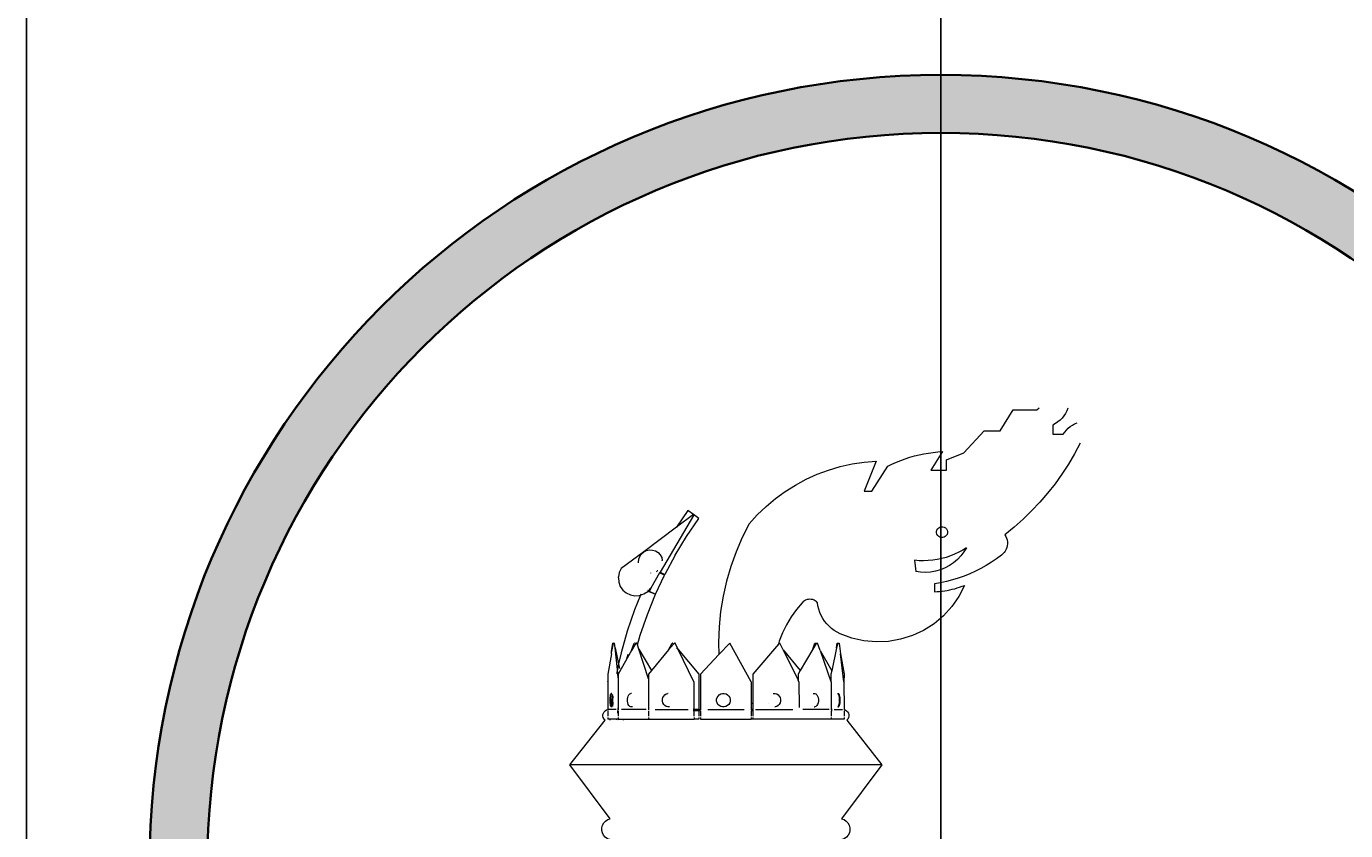
# Model space of a CAD drawing. Units: millimetres. Extents: x 446512 to 447461, y 70395 to 70610.
# Tile 30 of 39: x 447255 to 447300, y 70477 to 70505. Entities that reach past the tile are written whole.
import ezdxf

# ---------------------------------------------------------------- set-up
doc = ezdxf.new("R2010")
doc.units = ezdxf.units.MM
for name, color, linetype, lineweight in [('A-ANNO-DIMS', 2, 'Continuous', 18), ('A-FURN', 7, 'Continuous', 35), ('A-FURN-DECO', 8, 'Continuous', 13), ('A-FURN-PATT', 38, 'Continuous', 13)]:
    doc.layers.add(name, color=color, linetype=linetype, lineweight=lineweight)
doc.styles.get("Standard").update_dxf_attribs({"font": 'arial.ttf'})
doc.dimstyles.get("Standard").update_dxf_attribs({"dimtxt": 0.18, "dimasz": 0.18, "dimexe": 0.18, "dimexo": 0.0625, "dimgap": 0.09, "dimtad": 0, "dimtih": 1, "dimtoh": 1, "dimdec": 4, "dimzin": 0, "dimdsep": 46, "dimtxsty": 'Standard', "dimcen": 0.09, "dimadec": 0, "dimazin": 0, "dimtfac": 1, "dimtdec": 4, "dimtofl": 0, "dimtmove": 0, "dimatfit": 3, "dimfxl": 1, "dimtolj": 1, "dimtzin": 0, "dimarcsym": 0})

# ---------------------------------------------------------------- blocks, each defined once
blk = doc.blocks.new('DECO-SCULPTURE-BIRD')
for p, q in [((15.181, 34.03), (15.627, 34.749)), ((15.627, 34.749), (16.449, 34.749)), ((16.449, 34.749), (16.526, 34.819)), ((13.93, 33.268), (14.629, 34.03)), ((14.629, 34.03), (15.181, 34.03)), ((12.541, 33.233), (12.703, 33.261)), ((12.703, 33.261), (12.866, 33.283)), ((13.195, 33.309), (12.789, 32.676)), ((12.866, 33.283), (13.03, 33.299)), ((13.03, 33.299), (13.195, 33.309)), ((13.33, 33.029), (13.93, 33.268)), ((17.942, 33.598), (17.748, 33.234)), ((9.257, 32.674), (9.658, 32.793)), ((9.658, 32.793), (10.067, 32.884)), ((10.067, 32.884), (10.481, 32.948)), ((10.481, 32.948), (10.898, 32.983)), ((10.898, 32.983), (10.488, 31.945)), ((10.747, 31.945), (11.298, 32.806)), ((11.298, 32.806), (11.446, 32.878)), ((11.446, 32.878), (11.597, 32.946)), ((11.597, 32.946), (11.749, 33.008)), ((11.749, 33.008), (11.904, 33.064)), ((11.904, 33.064), (12.061, 33.115)), ((12.061, 33.115), (12.219, 33.16)), ((12.219, 33.16), (12.379, 33.199)), ((12.379, 33.199), (12.541, 33.233)), ((13.33, 32.676), (13.33, 33.029)), ((17.539, 32.879), (17.314, 32.533)), ((17.748, 33.234), (17.539, 32.879)), ((8.113, 32.157), (8.482, 32.355)), ((8.482, 32.355), (8.864, 32.528)), ((8.864, 32.528), (9.257, 32.674)), ((12.789, 32.676), (13.33, 32.676)), ((17.314, 32.533), (17.074, 32.198)), ((7.42, 31.689), (7.759, 31.935)), ((7.759, 31.935), (8.113, 32.157)), ((10.488, 31.945), (10.747, 31.945)), ((17.074, 32.198), (16.819, 31.874)), ((6.796, 31.131), (7.098, 31.42)), ((7.098, 31.42), (7.42, 31.689)), ((16.55, 31.562), (16.267, 31.262)), ((16.819, 31.874), (16.55, 31.562)), ((4.59, 31.11), (3.442, 29.152)), ((4.396, 31.274), (4.005, 30.703)), ((4.59, 31.141), (4.005, 30.703)), ((4.354, 30.38), (4.784, 31.008)), ((4.59, 31.141), (4.396, 31.274)), ((4.59, 31.11), (4.59, 31.141)), ((4.784, 31.008), (4.59, 31.141)), ((6.514, 30.821), (6.796, 31.131)), ((15.971, 30.975), (15.663, 30.701)), ((16.267, 31.262), (15.971, 30.975)), ((4.005, 30.703), (2.875, 29.852)), ((6.514, 30.821), (6.273, 30.344)), ((15.663, 30.701), (15.342, 30.442)), ((3.962, 29.736), (4.354, 30.38)), ((6.273, 30.344), (6.062, 29.854)), ((15.342, 30.442), (15.375, 30.385)), ((15.375, 30.385), (15.4, 30.324)), ((15.4, 30.324), (15.418, 30.261)), ((15.422, 30.065), (15.408, 30.001)), ((15.418, 30.261), (15.428, 30.196)), ((15.429, 30.13), (15.422, 30.065)), ((15.428, 30.196), (15.429, 30.13)), ((2.875, 29.852), (2.1, 29.278)), ((2.704, 29.597), (2.737, 29.696)), ((2.737, 29.696), (2.795, 29.783)), ((2.795, 29.783), (2.875, 29.852)), ((2.875, 29.852), (2.971, 29.899)), ((2.971, 29.899), (3.076, 29.921)), ((3.076, 29.921), (3.183, 29.915)), ((3.183, 29.915), (3.285, 29.883)), ((3.285, 29.883), (3.375, 29.827)), ((3.375, 29.827), (3.447, 29.75)), ((3.447, 29.75), (3.496, 29.657)), ((3.496, 29.657), (3.518, 29.556)), ((3.962, 29.736), (3.605, 29.071)), ((6.062, 29.854), (5.881, 29.351)), ((15.054, 29.609), (14.878, 29.491)), ((15.224, 29.735), (15.054, 29.609)), ((15.274, 29.778), (15.224, 29.735)), ((15.318, 29.827), (15.274, 29.778)), ((15.355, 29.881), (15.318, 29.827)), ((15.385, 29.939), (15.355, 29.881)), ((15.408, 30.001), (15.385, 29.939)), ((2.1, 29.278), (2.031, 29.139)), ((2.698, 29.494), (2.704, 29.597)), ((2.699, 29.49), (2.698, 29.494)), ((2.698, 29.476), (2.699, 29.49)), ((3.306, 29.18), (3.325, 29.171)), ((3.358, 29.194), (3.345, 29.201)), ((3.442, 29.152), (3.425, 29.125)), ((3.442, 29.152), (3.605, 29.071)), ((3.517, 29.541), (3.518, 29.556)), ((3.517, 29.541), (3.518, 29.538)), ((5.881, 29.351), (5.732, 28.838)), ((14.324, 29.181), (14.131, 29.094)), ((14.513, 29.277), (14.324, 29.181)), ((14.698, 29.38), (14.513, 29.277)), ((14.878, 29.491), (14.698, 29.38)), ((2.031, 29.139), (2.002, 28.989)), ((2.002, 28.958), (2.002, 28.989)), ((2.002, 28.958), (2.013, 28.805)), ((2.013, 28.805), (2.066, 28.66)), ((3.425, 29.125), (3.119, 28.602)), ((3.287, 28.392), (3.593, 29.046)), ((3.593, 29.046), (3.425, 29.125)), ((5.732, 28.838), (5.615, 28.317)), ((13.121, 28.783), (12.912, 28.746)), ((12.912, 28.746), (12.912, 28.476)), ((13.328, 28.828), (13.121, 28.783)), ((13.532, 28.882), (13.328, 28.828)), ((13.735, 28.944), (13.532, 28.882)), ((13.934, 29.015), (13.735, 28.944)), ((13.947, 28.695), (13.752, 28.315)), ((13.864, 28.663), (13.947, 28.695)), ((14.131, 29.094), (13.934, 29.015)), ((2.066, 28.66), (2.155, 28.533)), ((2.155, 28.533), (2.275, 28.433)), ((2.275, 28.433), (2.419, 28.366)), ((2.419, 28.366), (2.575, 28.337)), ((2.766, 28.36), (2.561, 27.852)), ((2.575, 28.337), (2.733, 28.349)), ((2.733, 28.349), (2.766, 28.36)), ((2.766, 28.36), (2.883, 28.399)), ((2.781, 28.395), (2.766, 28.36)), ((2.883, 28.399), (3.015, 28.486)), ((3.002, 27.688), (3.284, 28.387)), ((3.005, 28.509), (3.027, 28.499)), ((3.015, 28.486), (3.027, 28.499)), ((3.036, 28.509), (3.019, 28.518)), ((3.027, 28.499), (3.036, 28.509)), ((3.027, 28.499), (3.284, 28.387)), ((3.036, 28.509), (3.119, 28.602)), ((3.036, 28.509), (3.287, 28.392)), ((3.074, 28.492), (3.069, 28.481)), ((3.152, 28.659), (3.074, 28.492)), ((5.615, 28.317), (5.531, 27.79)), ((12.912, 28.476), (13.001, 28.48)), ((13.001, 28.48), (13.089, 28.487)), ((13.089, 28.487), (13.177, 28.496)), ((13.177, 28.496), (13.265, 28.508)), ((13.265, 28.508), (13.352, 28.523)), ((13.352, 28.523), (13.439, 28.54)), ((13.439, 28.54), (13.525, 28.559)), ((13.752, 28.315), (13.509, 27.964)), ((13.525, 28.559), (13.611, 28.581)), ((13.611, 28.581), (13.696, 28.606)), ((13.696, 28.606), (13.781, 28.633)), ((13.781, 28.633), (13.864, 28.663)), ((2.561, 27.852), (2.308, 27.114)), ((5.531, 27.79), (5.479, 27.259)), ((8.147, 27.859), (7.968, 27.605)), ((8.346, 28.098), (8.147, 27.859)), ((8.382, 28.133), (8.346, 28.098)), ((8.422, 28.162), (8.382, 28.133)), ((8.466, 28.185), (8.422, 28.162)), ((8.513, 28.202), (8.466, 28.185)), ((8.561, 28.212), (8.513, 28.202)), ((8.611, 28.216), (8.561, 28.212)), ((8.66, 28.212), (8.611, 28.216)), ((8.709, 28.202), (8.66, 28.212)), ((8.756, 28.185), (8.709, 28.202)), ((8.799, 28.162), (8.756, 28.185)), ((8.84, 28.133), (8.799, 28.162)), ((8.875, 28.098), (8.84, 28.133)), ((8.892, 27.984), (8.875, 28.098)), ((8.919, 27.871), (8.892, 27.984)), ((8.956, 27.761), (8.919, 27.871)), ((13.509, 27.964), (13.223, 27.648)), ((2.757, 26.974), (3.002, 27.688)), ((7.808, 27.338), (7.671, 27.059)), ((7.968, 27.605), (7.808, 27.338)), ((9.002, 27.655), (8.956, 27.761)), ((9.057, 27.553), (9.002, 27.655)), ((9.121, 27.456), (9.057, 27.553)), ((9.193, 27.366), (9.121, 27.456)), ((9.273, 27.282), (9.193, 27.366)), ((12.897, 27.372), (12.537, 27.142)), ((13.223, 27.648), (12.897, 27.372)), ((2.308, 27.114), (2.095, 26.364)), ((2.662, 26.638), (2.757, 26.974)), ((5.479, 27.259), (5.46, 26.725)), ((7.671, 27.059), (7.556, 26.77)), ((9.359, 27.205), (9.273, 27.282)), ((9.452, 27.136), (9.359, 27.205)), ((9.551, 27.075), (9.452, 27.136)), ((9.654, 27.023), (9.551, 27.075)), ((10.055, 26.875), (9.654, 27.023)), ((10.471, 26.78), (10.055, 26.875)), ((12.15, 26.961), (11.743, 26.833)), ((12.537, 27.142), (12.15, 26.961)), ((1.77, 26.41), (1.808, 26.703)), ((1.827, 26.703), (1.77, 26.41)), ((1.827, 26.703), (1.808, 26.703)), ((1.827, 26.703), (1.873, 26.703)), ((1.89, 26.535), (1.873, 26.703)), ((1.89, 26.535), (2.01, 25.987)), ((1.967, 25.795), (1.89, 26.535)), ((2.459, 26.45), (1.998, 25.636)), ((2.459, 26.45), (2.547, 26.703)), ((2.603, 26.703), (2.459, 26.45)), ((2.558, 26.703), (2.547, 26.703)), ((2.64, 26.703), (2.603, 26.703)), ((2.662, 26.638), (2.64, 26.703)), ((2.709, 26.493), (2.662, 26.638)), ((2.709, 26.493), (3.149, 25.76)), ((3.046, 25.467), (2.709, 26.493)), ((3.737, 26.466), (3.149, 25.76)), ((3.737, 26.466), (3.854, 26.703)), ((3.905, 26.667), (3.737, 26.466)), ((3.875, 26.703), (3.854, 26.703)), ((3.875, 26.703), (3.905, 26.667)), ((3.935, 26.703), (3.905, 26.667)), ((3.957, 26.703), (3.935, 26.703)), ((4.064, 26.48), (3.957, 26.703)), ((4.013, 26.541), (4.064, 26.48)), ((4.064, 26.48), (4.783, 25.636)), ((4.603, 25.364), (4.064, 26.48)), ((5.46, 26.725), (5.471, 26.308)), ((5.845, 26.703), (5.471, 26.308)), ((6.58, 25.364), (5.845, 26.703)), ((7.523, 26.665), (6.643, 25.636)), ((7.523, 26.665), (7.514, 26.636)), ((7.526, 26.673), (7.523, 26.665)), ((7.523, 26.665), (7.531, 26.655)), ((7.556, 26.77), (7.526, 26.673)), ((7.551, 26.703), (7.526, 26.673)), ((7.551, 26.703), (7.572, 26.703)), ((7.688, 26.466), (7.572, 26.703)), ((7.688, 26.466), (8.277, 25.76)), ((7.688, 26.466), (8.203, 25.423)), ((8.717, 26.493), (8.277, 25.76)), ((8.717, 26.493), (8.786, 26.703)), ((8.833, 26.686), (8.717, 26.493)), ((8.786, 26.703), (8.823, 26.703)), ((8.823, 26.703), (8.833, 26.686)), ((8.843, 26.703), (8.833, 26.686)), ((8.843, 26.703), (8.879, 26.703)), ((8.967, 26.45), (8.879, 26.703)), ((8.967, 26.45), (9.364, 25.75)), ((8.967, 26.45), (9.339, 25.38)), ((9.536, 26.535), (9.364, 25.75)), ((9.536, 26.535), (9.553, 26.703)), ((9.573, 26.703), (9.536, 26.535)), ((9.553, 26.703), (9.573, 26.703)), ((9.573, 26.703), (9.618, 26.703)), ((9.618, 26.703), (9.665, 26.337)), ((10.896, 26.742), (10.471, 26.78)), ((11.323, 26.759), (10.896, 26.742)), ((11.743, 26.833), (11.323, 26.759)), ((1.761, 26.337), (1.636, 25.636)), ((1.761, 26.337), (1.77, 26.41)), ((2.01, 25.987), (1.967, 25.795)), ((2.095, 26.364), (2.01, 25.987)), ((2.01, 25.987), (2.045, 25.829)), ((5.471, 26.308), (4.835, 25.636)), ((9.665, 26.337), (9.79, 25.636)), ((9.789, 25.364), (9.665, 26.337)), ((1.636, 25.636), (1.639, 25.38)), ((1.967, 25.795), (1.935, 25.655)), ((1.998, 25.499), (1.967, 25.795)), ((1.998, 25.636), (1.998, 25.499)), ((3.149, 25.76), (3.046, 25.636)), ((3.046, 25.636), (3.046, 25.467)), ((4.783, 25.636), (4.783, 24.41)), ((4.835, 25.636), (4.835, 24.41)), ((6.643, 25.636), (6.643, 24.617)), ((8.277, 25.76), (8.203, 25.636)), ((8.203, 25.636), (8.203, 25.423)), ((9.364, 25.75), (9.339, 25.636)), ((9.339, 25.636), (9.339, 25.38)), ((9.79, 25.636), (9.789, 25.364)), ((1.637, 25.364), (1.635, 24.407)), ((1.637, 25.364), (1.639, 25.38)), ((1.998, 25.499), (1.998, 24.41)), ((3.046, 25.467), (3.046, 24.397)), ((4.603, 25.364), (4.61, 24.41)), ((6.58, 25.364), (6.586, 24.617)), ((8.232, 25.364), (8.203, 25.423)), ((8.232, 25.364), (8.239, 24.482)), ((9.344, 25.364), (9.339, 25.38)), ((9.344, 25.364), (9.349, 24.41)), ((9.789, 25.364), (9.79, 24.407)), ((6.643, 24.617), (6.586, 24.617)), ((6.586, 24.617), (6.588, 24.41)), ((6.663, 24.617), (6.643, 24.617)), ((6.643, 24.617), (6.643, 24.41)), ((1.467, 24.182), (1.468, 24.235)), ((1.48, 24.13), (1.467, 24.182)), ((1.468, 24.235), (1.483, 24.287)), ((1.483, 24.287), (1.51, 24.333)), ((1.51, 24.333), (1.549, 24.371)), ((1.549, 24.371), (1.595, 24.397)), ((1.595, 24.397), (1.635, 24.407)), ((1.635, 24.407), (1.648, 24.41)), ((1.635, 24.407), (1.635, 24.397)), ((1.635, 24.371), (1.635, 24.182)), ((1.648, 24.41), (1.657, 24.41)), ((1.648, 24.41), (1.651, 24.41)), ((1.923, 24.41), (1.657, 24.41)), ((1.998, 24.41), (1.967, 24.41)), ((1.977, 24.371), (1.967, 24.29)), ((1.998, 24.367), (1.967, 24.367)), ((1.998, 24.556), (1.98, 24.397)), ((1.998, 24.41), (1.998, 24.397)), ((1.998, 24.371), (1.998, 24.367)), ((1.998, 24.367), (1.998, 24.182)), ((2.958, 24.41), (2.109, 24.41)), ((3.046, 24.371), (3.046, 24.182)), ((4.61, 24.41), (4.588, 24.41)), ((4.611, 24.367), (4.588, 24.367)), ((4.61, 24.41), (4.611, 24.397)), ((4.783, 24.41), (4.61, 24.41)), ((4.611, 24.371), (4.611, 24.367)), ((4.611, 24.367), (4.612, 24.182)), ((4.783, 24.367), (4.611, 24.367)), ((4.783, 24.41), (4.835, 24.41)), ((4.783, 24.41), (4.783, 24.397)), ((4.783, 24.371), (4.783, 24.367)), ((4.783, 24.367), (4.783, 24.182)), ((4.835, 24.367), (4.783, 24.367)), ((4.835, 24.41), (4.835, 24.397)), ((4.835, 24.371), (4.835, 24.367)), ((4.835, 24.367), (4.835, 24.182)), ((6.588, 24.41), (6.588, 24.397)), ((6.643, 24.41), (6.588, 24.41)), ((6.588, 24.371), (6.588, 24.367)), ((6.588, 24.367), (6.59, 24.182)), ((6.643, 24.367), (6.588, 24.367)), ((6.663, 24.41), (6.643, 24.41)), ((6.643, 24.41), (6.643, 24.397)), ((6.643, 24.371), (6.643, 24.367)), ((6.663, 24.367), (6.643, 24.367)), ((6.643, 24.367), (6.643, 24.182)), ((6.737, 24.41), (8.029, 24.41)), ((9.272, 24.41), (8.372, 24.41)), ((9.384, 24.41), (9.349, 24.41)), ((9.349, 24.41), (9.35, 24.397)), ((9.35, 24.371), (9.35, 24.367)), ((9.384, 24.367), (9.35, 24.367)), ((9.35, 24.367), (9.351, 24.182)), ((9.445, 24.41), (9.742, 24.41)), ((9.79, 24.407), (9.83, 24.397)), ((9.79, 24.407), (9.79, 24.397)), ((9.79, 24.371), (9.79, 24.182)), ((9.83, 24.397), (9.877, 24.371)), ((9.877, 24.371), (9.916, 24.333)), ((9.916, 24.333), (9.943, 24.287)), ((9.943, 24.287), (9.958, 24.235)), ((9.959, 24.182), (9.946, 24.13)), ((9.958, 24.235), (9.959, 24.182)), ((0.327, 22.505), (1.544, 24.044)), ((1.507, 24.083), (1.48, 24.13)), ((1.544, 24.044), (1.507, 24.083)), ((1.635, 24.13), (1.635, 24.083)), ((1.639, 24.083), (1.635, 24.083)), ((1.707, 24.083), (1.635, 24.083)), ((1.704, 24.059), (1.703, 24.044)), ((1.707, 24.083), (1.704, 24.059)), ((1.998, 24.083), (1.707, 24.083)), ((1.944, 24.083), (1.939, 24.044)), ((1.998, 24.13), (1.998, 24.083)), ((1.998, 24.083), (2.18, 24.083)), ((2.176, 24.044), (2.18, 24.083)), ((2.18, 24.083), (3.049, 24.083)), ((3.046, 24.13), (3.049, 24.083)), ((3.049, 24.083), (4.613, 24.083)), ((4.613, 24.13), (4.613, 24.083)), ((4.783, 24.083), (4.613, 24.083)), ((4.783, 24.13), (4.783, 24.083)), ((4.835, 24.13), (4.835, 24.083)), ((4.835, 24.083), (6.591, 24.083)), ((6.59, 24.13), (6.591, 24.083)), ((6.643, 24.083), (6.591, 24.083)), ((6.643, 24.13), (6.643, 24.083)), ((9.351, 24.083), (6.643, 24.083)), ((9.351, 24.13), (9.351, 24.083)), ((9.79, 24.083), (9.351, 24.083)), ((9.79, 24.13), (9.79, 24.083)), ((9.919, 24.083), (9.882, 24.044)), ((9.882, 24.044), (11.099, 22.505)), ((9.946, 24.13), (9.919, 24.083)), ((1.72, 20.641), (0.327, 22.505)), ((11.099, 22.505), (0.327, 22.505)), ((11.099, 22.505), (9.706, 20.641)), ((1.455, 20.417), (1.498, 20.496)), ((1.498, 20.496), (1.56, 20.562)), ((1.56, 20.562), (1.635, 20.611)), ((1.635, 20.611), (1.72, 20.641)), ((9.706, 20.641), (9.791, 20.611)), ((9.791, 20.611), (9.866, 20.562)), ((9.866, 20.562), (9.927, 20.496)), ((9.927, 20.496), (9.971, 20.417)), ((1.431, 20.239), (1.432, 20.329)), ((1.451, 20.152), (1.431, 20.239)), ((1.432, 20.329), (1.455, 20.417)), ((1.492, 20.071), (1.451, 20.152)), ((1.551, 20.003), (1.492, 20.071)), ((9.934, 20.071), (9.874, 20.003)), ((9.975, 20.152), (9.934, 20.071)), ((9.971, 20.417), (9.994, 20.329)), ((9.995, 20.239), (9.975, 20.152)), ((9.994, 20.329), (9.995, 20.239)), ((1.48, 18.035), (1.609, 19.909)), ((1.625, 19.952), (1.551, 20.003)), ((1.799, 19.909), (1.609, 19.909)), ((1.709, 19.92), (1.625, 19.952)), ((1.648, 18.028), (2.417, 19.746)), ((1.799, 19.909), (1.709, 19.92)), ((1.799, 19.909), (2.323, 19.909)), ((2.323, 19.909), (2.359, 19.909)), ((2.364, 19.896), (2.323, 19.909)), ((2.364, 19.896), (2.359, 19.909)), ((2.359, 19.909), (4.323, 19.909)), ((2.417, 19.746), (2.364, 19.896)), ((2.508, 19.49), (2.417, 19.746)), ((3.245, 18.169), (4.419, 19.866)), ((3.386, 17.993), (4.578, 19.714)), ((4.323, 19.909), (4.479, 19.909)), ((4.419, 19.866), (4.323, 19.909)), ((4.479, 19.866), (4.479, 19.909)), ((6.726, 19.909), (4.479, 19.909)), ((4.578, 19.714), (4.479, 19.866)), ((5.313, 18.586), (4.578, 19.714)), ((6.112, 18.612), (6.893, 19.784)), ((6.112, 18.284), (6.985, 19.65)), ((6.922, 19.907), (6.726, 19.909)), ((6.893, 19.784), (6.878, 19.805)), ((6.985, 19.65), (6.893, 19.784)), ((6.922, 19.907), (6.926, 19.909)), ((6.926, 19.909), (6.936, 19.909)), ((8.957, 19.909), (6.936, 19.909)), ((8.126, 17.993), (6.985, 19.65)), ((8.239, 18.093), (8.898, 19.762)), ((8.405, 18.035), (8.967, 19.615)), ((8.898, 19.762), (8.95, 19.895)), ((8.967, 19.615), (8.898, 19.762)), ((8.95, 19.895), (8.999, 19.909)), ((8.95, 19.895), (8.957, 19.909)), ((8.957, 19.909), (8.999, 19.909)), ((9.727, 17.993), (8.967, 19.615)), ((8.999, 19.909), (9.627, 19.909)), ((9.716, 19.92), (9.627, 19.909)), ((9.807, 19.907), (9.627, 19.909)), ((9.801, 19.952), (9.716, 19.92)), ((9.874, 20.003), (9.801, 19.952)), ((9.814, 19.909), (9.807, 19.907)), ((9.816, 19.893), (9.814, 19.909)), ((9.974, 18.035), (9.816, 19.893)), ((9.876, 18.035), (9.816, 19.893)), ((1.771, 17.993), (2.508, 19.49)), ((3.027, 18.035), (2.508, 19.49)), ((5.313, 11.612), (5.313, 18.586)), ((5.7, 17.993), (5.313, 18.586)), ((5.812, 18.161), (6.112, 18.612)), ((5.995, 18.101), (6.112, 18.284)), ((6.112, 18.612), (6.112, 18.655)), ((6.112, 18.284), (6.112, 18.612)), ((6.112, 11.612), (6.112, 18.284)), ((3.123, 17.993), (3.027, 18.035)), ((3.123, 17.993), (3.245, 18.169)), ((3.299, 18.035), (3.245, 18.169)), ((3.386, 17.993), (3.299, 18.035)), ((5.7, 17.993), (5.812, 18.161)), ((5.812, 18.161), (5.798, 18.182)), ((5.816, 18.155), (5.812, 18.161)), ((0, 0), (0, 11.612)), ((0, 11.612), (5.313, 11.612)), ((6.112, 11.612), (5.313, 11.612)), ((6.112, 11.612), (11.751, 11.612)), ((11.751, 0), (11.751, 11.612)), ((0, 0), (11.751, 0))]:
    blk.add_line(p, q)
blk = doc.blocks.new('*D62')
at = {"layer": 'A-ANNO-DIMS', "color": 0, "lineweight": -2, "transparency": 16777216}
for p, q in [((447254.943, 70456.952), (447254.943, 70610.145)), ((447286.509, 70475.943), (447286.509, 70610.145)), ((447255.123, 70609.965), (447270.262, 70609.965)), ((447286.329, 70609.965), (447271.189, 70609.965))]:
    blk.add_line(p, q, dxfattribs=at)
at = {"layer": 'A-ANNO-DIMS', "color": 0, "transparency": 16777216}
for points in [[(447255.123, 70609.995), (447255.123, 70609.935), (447254.943, 70609.965)], [(447286.329, 70609.995), (447286.329, 70609.935), (447286.509, 70609.965)]]:
    blk.add_solid(points, dxfattribs=at)
at = {"layer": 'Defpoints', "color": 0, "transparency": 16777216}
for p in [(447286.509, 70609.965), (447286.509, 70475.881), (447254.943, 70456.89)]:
    blk.add_point(p, dxfattribs=at)
at = {"layer": 'A-ANNO-DIMS', "color": 0, "transparency": 16777216, "insert": (447270.726, 70609.965), "char_height": 0.18, "attachment_point": 5}
blk.add_mtext('\\A1;31.566', dxfattribs=at)
blk = doc.blocks.new('*D63')
at = {"layer": 'A-ANNO-DIMS', "color": 0, "lineweight": -2, "transparency": 16777216}
for p, q in [((447286.509, 70475.943), (447286.509, 70610.145)), ((447340.049, 70506.612), (447340.049, 70610.145)), ((447286.689, 70609.965), (447312.886, 70609.965)), ((447339.869, 70609.965), (447313.672, 70609.965))]:
    blk.add_line(p, q, dxfattribs=at)
at = {"layer": 'A-ANNO-DIMS', "color": 0, "transparency": 16777216}
for points in [[(447286.689, 70609.995), (447286.689, 70609.935), (447286.509, 70609.965)], [(447339.869, 70609.995), (447339.869, 70609.935), (447340.049, 70609.965)]]:
    blk.add_solid(points, dxfattribs=at)
at = {"layer": 'Defpoints', "color": 0, "transparency": 16777216}
for p in [(447340.049, 70609.965), (447340.049, 70506.55), (447286.509, 70475.881)]:
    blk.add_point(p, dxfattribs=at)
at = {"layer": 'A-ANNO-DIMS', "color": 0, "transparency": 16777216, "insert": (447313.279, 70609.965), "char_height": 0.18, "attachment_point": 5}
blk.add_mtext('\\A1;53.54', dxfattribs=at)

msp = doc.modelspace()

# ---------------------------------------------------------------- hatches: boundary and pattern name
at = {"layer": 'A-FURN-PATT'}
h = msp.add_hatch(color=256, dxfattribs=at)
h.dxf.hatch_style = 1
h.paths.add_polyline_path([(447259.1901, 70475.8806, 0.1945594), (447266.8704, 70456.89), (447269.7639, 70456.89, -0.2152771), (447261.1901, 70475.8806, -1), (447311.827, 70475.8806, -0.2152771), (447303.2532, 70456.89), (447306.1467, 70456.89, 0.1945594), (447313.827, 70475.8806, 1)])
h.paths.add_polyline_path([(447301.2097, 70452.855), (447297.037, 70452.855, -0.2177821), (447275.9801, 70452.855), (447271.8074, 70452.855, 0.2920128)])
h.paths.add_polyline_path([(447269.7639, 70456.89), (447266.8704, 70456.89, 0.0585505), (447271.8074, 70452.855), (447275.9801, 70452.855, -0.0735735)])
h.paths.add_polyline_path([(447306.1467, 70456.89), (447303.2532, 70456.89, -0.0735735), (447297.037, 70452.855), (447301.2097, 70452.855, 0.0585505)])

# ---------------------------------------------------------------- linework, layer by layer
at = {"layer": 'A-FURN'}
for radius in [27.3185, 25.3185]:
    msp.add_circle((447286.5086, 70475.8806), radius, dxfattribs=at)
at = {"layer": 'A-FURN-DECO'}
for p, q in [((447290.851, 70491.6087), (447290.8051, 70491.5208)), ((447290.8884, 70491.7006), (447290.851, 70491.6087)), ((447290.4647, 70491.166), (447290.3787, 70491.1165)), ((447290.5456, 70491.2234), (447290.4647, 70491.166)), ((447290.6208, 70491.2882), (447290.5456, 70491.2234)), ((447290.6895, 70491.3598), (447290.6208, 70491.2882)), ((447290.7511, 70491.4375), (447290.6895, 70491.3598)), ((447290.8051, 70491.5208), (447290.7511, 70491.4375)), ((447291.0473, 70491.1147), (447291.1266, 70491.1574)), ((447291.1266, 70491.1574), (447291.2098, 70491.1923)), ((447290.3787, 70491.1165), (447290.3787, 70490.7992)), ((447290.3787, 70490.7992), (447290.7313, 70490.7992)), ((447290.7313, 70490.7992), (447290.7816, 70490.874)), ((447290.7816, 70490.874), (447290.839, 70490.9435)), ((447290.839, 70490.9435), (447290.9028, 70491.0072)), ((447290.9028, 70491.0072), (447290.9724, 70491.0644)), ((447290.9724, 70491.0644), (447291.0473, 70491.1147)), ((447286.3616, 70487.4435), (447286.3746, 70487.4908)), ((447286.3746, 70487.4908), (447286.3993, 70487.5332)), ((447286.3993, 70487.5332), (447286.4342, 70487.5677)), ((447286.4342, 70487.5677), (447286.4768, 70487.592)), ((447286.4768, 70487.592), (447286.5243, 70487.6045)), ((447286.5243, 70487.6045), (447286.5734, 70487.6042)), ((447286.5734, 70487.6042), (447286.6207, 70487.5913)), ((447286.6207, 70487.5913), (447286.6631, 70487.5665)), ((447286.6631, 70487.5665), (447286.6976, 70487.5316)), ((447286.6976, 70487.5316), (447286.722, 70487.489)), ((447286.722, 70487.489), (447286.7344, 70487.4415)), ((447286.3614, 70487.3944), (447286.3616, 70487.4435)), ((447286.3738, 70487.3469), (447286.3614, 70487.3944)), ((447286.3981, 70487.3043), (447286.3738, 70487.3469)), ((447286.4327, 70487.2694), (447286.3981, 70487.3043)), ((447286.475, 70487.2446), (447286.4327, 70487.2694)), ((447286.5224, 70487.2317), (447286.475, 70487.2446)), ((447286.5715, 70487.2314), (447286.5224, 70487.2317)), ((447286.6189, 70487.2439), (447286.5715, 70487.2314)), ((447286.6616, 70487.2682), (447286.6189, 70487.2439)), ((447286.6965, 70487.3027), (447286.6616, 70487.2682)), ((447286.7212, 70487.3451), (447286.6965, 70487.3027)), ((447286.7342, 70487.3925), (447286.7212, 70487.3451)), ((447286.7344, 70487.4415), (447286.7342, 70487.3925)), ((447286.8361, 70486.5999), (447286.6874, 70486.5496)), ((447286.9815, 70486.6589), (447286.8361, 70486.5999)), ((447287.1233, 70486.7263), (447286.9815, 70486.6589)), ((447287.1977, 70486.6015), (447287.0784, 70486.4764)), ((447287.2608, 70486.802), (447287.1233, 70486.7263)), ((447287.3032, 70486.7383), (447287.1977, 70486.6015)), ((447287.3936, 70486.8856), (447287.2608, 70486.802)), ((447287.3936, 70486.8856), (447287.3032, 70486.7383)), ((447285.7572, 70486.4369), (447285.6008, 70486.4503)), ((447285.6008, 70486.4503), (447285.6393, 70486.0599)), ((447285.9141, 70486.4328), (447285.7572, 70486.4369)), ((447286.071, 70486.4378), (447285.9141, 70486.4328)), ((447286.2273, 70486.4521), (447286.071, 70486.4378)), ((447286.3825, 70486.4755), (447286.2273, 70486.4521)), ((447286.4916, 70486.1204), (447286.3256, 70486.0724)), ((447286.536, 70486.5081), (447286.3825, 70486.4755)), ((447286.6516, 70486.1857), (447286.4916, 70486.1204)), ((447286.6874, 70486.5496), (447286.536, 70486.5081)), ((447286.8038, 70486.2674), (447286.6516, 70486.1857)), ((447286.9467, 70486.3647), (447286.8038, 70486.2674)), ((447287.0784, 70486.4764), (447286.9467, 70486.3647)), ((447276.4886, 70486.0201), (447276.4802, 70486.0023)), ((447285.8104, 70486.0358), (447285.6393, 70486.0599)), ((447285.9831, 70486.0298), (447285.8104, 70486.0358)), ((447286.1555, 70486.0421), (447285.9831, 70486.0298)), ((447286.3256, 70486.0724), (447286.1555, 70486.0421)), ((447275.6982, 70483.1959), (447275.6623, 70483.037)), ((447275.0933, 70481.653), (447275.0963, 70481.7122)), ((447275.0933, 70481.5917), (447275.0933, 70481.653)), ((447275.0962, 70481.5324), (447275.0933, 70481.5917)), ((447275.0963, 70481.7122), (447275.1021, 70481.7653)), ((447275.1021, 70481.7653), (447275.1104, 70481.8086)), ((447275.1104, 70481.8086), (447275.1204, 70481.8391)), ((447275.1163, 70481.5917), (447275.1164, 70481.653)), ((447275.1193, 70481.5324), (447275.1163, 70481.5917)), ((447275.1164, 70481.653), (447275.1194, 70481.7122)), ((447275.1194, 70481.7122), (447275.1252, 70481.7653)), ((447275.1204, 70481.8391), (447275.1316, 70481.8548)), ((447275.1252, 70481.7653), (447275.1334, 70481.8086)), ((447275.1547, 70481.8548), (447275.1316, 70481.8548)), ((447275.1563, 70481.5904), (447275.1333, 70481.4356)), ((447275.1334, 70481.8086), (447275.1435, 70481.8391)), ((447275.1435, 70481.8391), (447275.1547, 70481.8548)), ((447275.1599, 70481.7111), (447275.1563, 70481.6518)), ((447275.1563, 70481.6518), (447275.1563, 70481.5904)), ((447275.1563, 70481.5904), (447275.16, 70481.5312)), ((447275.167, 70481.7643), (447275.1599, 70481.7111)), ((447275.168, 70481.724), (447275.1599, 70481.7111)), ((447275.177, 70481.8078), (447275.167, 70481.7643)), ((447275.167, 70481.7643), (447275.168, 70481.724)), ((447275.1828, 70481.8224), (447275.177, 70481.8078)), ((447275.1841, 70481.8185), (447275.177, 70481.8078)), ((447275.1828, 70481.7111), (447275.1791, 70481.6518)), ((447275.1791, 70481.6518), (447275.1792, 70481.5904)), ((447275.1792, 70481.5904), (447275.1829, 70481.5312)), ((447275.1898, 70481.7643), (447275.1828, 70481.7111)), ((447275.1931, 70481.7784), (447275.1898, 70481.7643)), ((447275.6886, 70481.5917), (447275.6887, 70481.653)), ((447275.698, 70481.5324), (447275.6886, 70481.5917)), ((447275.6887, 70481.653), (447275.6983, 70481.7122)), ((447275.6983, 70481.7122), (447275.7168, 70481.7653)), ((447275.7168, 70481.7653), (447275.7428, 70481.8086)), ((447275.7428, 70481.8086), (447275.7747, 70481.8391)), ((447275.7747, 70481.8391), (447275.8102, 70481.8548)), ((447275.829, 70481.8548), (447275.8102, 70481.8548)), ((447276.9017, 70481.5917), (447276.9018, 70481.653)), ((447276.9155, 70481.5324), (447276.9017, 70481.5917)), ((447276.9018, 70481.653), (447276.9159, 70481.7122)), ((447276.9159, 70481.7122), (447276.943, 70481.7653)), ((447276.943, 70481.7653), (447276.9813, 70481.8086)), ((447276.9813, 70481.8086), (447277.0281, 70481.8391)), ((447277.0281, 70481.8391), (447277.0803, 70481.8548)), ((447277.0915, 70481.8548), (447277.0803, 70481.8548)), ((447278.769, 70481.5917), (447278.7691, 70481.653)), ((447278.7847, 70481.5324), (447278.769, 70481.5917)), ((447278.7691, 70481.653), (447278.7852, 70481.7122)), ((447278.7852, 70481.7122), (447278.816, 70481.7653)), ((447278.816, 70481.7653), (447278.8595, 70481.8086)), ((447278.8595, 70481.8086), (447278.9127, 70481.8391)), ((447278.9127, 70481.8391), (447278.972, 70481.8548)), ((447278.972, 70481.8548), (447279.0333, 70481.8546)), ((447279.0333, 70481.8546), (447279.0926, 70481.8386)), ((447279.0926, 70481.8386), (447279.1456, 70481.8078)), ((447279.1456, 70481.8078), (447279.1889, 70481.7643)), ((447279.1889, 70481.7643), (447279.2194, 70481.7111)), ((447279.235, 70481.5904), (447279.2189, 70481.5312)), ((447279.2194, 70481.7111), (447279.2351, 70481.6518)), ((447279.2351, 70481.6518), (447279.235, 70481.5904)), ((447280.7235, 70481.8548), (447280.7338, 70481.8548)), ((447280.7338, 70481.8548), (447280.789, 70481.8546)), ((447280.789, 70481.8546), (447280.8422, 70481.8386)), ((447280.8422, 70481.8386), (447280.8899, 70481.8078)), ((447280.8899, 70481.8078), (447280.9289, 70481.7643)), ((447280.9289, 70481.7643), (447280.9563, 70481.7111)), ((447280.9703, 70481.5904), (447280.9559, 70481.5312)), ((447280.9563, 70481.7111), (447280.9705, 70481.6518)), ((447280.9705, 70481.6518), (447280.9703, 70481.5904)), ((447282.0968, 70481.8548), (447282.115, 70481.8548)), ((447282.115, 70481.8548), (447282.1539, 70481.8546)), ((447282.1539, 70481.8546), (447282.1914, 70481.8386)), ((447282.1914, 70481.8386), (447282.225, 70481.8078)), ((447282.225, 70481.8078), (447282.2524, 70481.7643)), ((447282.2524, 70481.7643), (447282.2717, 70481.7111)), ((447282.2816, 70481.5904), (447282.2714, 70481.5312)), ((447282.2717, 70481.7111), (447282.2817, 70481.6518)), ((447282.2817, 70481.6518), (447282.2816, 70481.5904)), ((447282.9358, 70481.8548), (447282.95, 70481.8546)), ((447282.95, 70481.8546), (447282.9587, 70481.8548)), ((447282.95, 70481.8546), (447282.9637, 70481.8386)), ((447282.9587, 70481.8548), (447282.9729, 70481.8546)), ((447282.9637, 70481.8386), (447282.976, 70481.8078)), ((447282.9729, 70481.8546), (447282.9866, 70481.8386)), ((447282.976, 70481.8078), (447282.9861, 70481.7643)), ((447282.9861, 70481.7643), (447282.9931, 70481.7111)), ((447282.9866, 70481.8386), (447282.9989, 70481.8078)), ((447282.9968, 70481.5904), (447282.993, 70481.5312)), ((447282.9931, 70481.7111), (447282.9968, 70481.6518)), ((447282.9968, 70481.6518), (447282.9968, 70481.5904)), ((447282.9989, 70481.8078), (447283.0089, 70481.7643)), ((447283.0089, 70481.7643), (447283.016, 70481.7111)), ((447283.0196, 70481.5904), (447283.0159, 70481.5312)), ((447283.016, 70481.7111), (447283.0197, 70481.6518)), ((447283.0197, 70481.6518), (447283.0196, 70481.5904)), ((447275.102, 70481.4791), (447275.0962, 70481.5324)), ((447275.1102, 70481.4356), (447275.102, 70481.4791)), ((447275.1202, 70481.4048), (447275.1102, 70481.4356)), ((447275.1251, 70481.4791), (447275.1193, 70481.5324)), ((447275.1314, 70481.3888), (447275.1202, 70481.4048)), ((447275.1333, 70481.4356), (447275.1251, 70481.4791)), ((447275.143, 70481.3886), (447275.1314, 70481.3888)), ((447275.1433, 70481.4048), (447275.1333, 70481.4356)), ((447275.1545, 70481.3888), (447275.143, 70481.3886)), ((447275.1545, 70481.3888), (447275.1433, 70481.4048)), ((447275.1661, 70481.3886), (447275.1545, 70481.3888)), ((447275.16, 70481.5312), (447275.1672, 70481.4781)), ((447275.1672, 70481.4781), (447275.1772, 70481.4349)), ((447275.1772, 70481.4349), (447275.1828, 70481.4211)), ((447275.1829, 70481.5312), (447275.19, 70481.4781)), ((447275.19, 70481.4781), (447275.1931, 70481.465)), ((447275.7163, 70481.4791), (447275.698, 70481.5324)), ((447275.7422, 70481.4356), (447275.7163, 70481.4791)), ((447275.774, 70481.4048), (447275.7422, 70481.4356)), ((447275.8095, 70481.3888), (447275.774, 70481.4048)), ((447275.8462, 70481.3886), (447275.8095, 70481.3888)), ((447275.8651, 70481.3886), (447275.8462, 70481.3886)), ((447276.6505, 70481.2999), (447277.7804, 70481.2999)), ((447276.9424, 70481.4791), (447276.9155, 70481.5324)), ((447276.9804, 70481.4356), (447276.9424, 70481.4791)), ((447277.0271, 70481.4048), (447276.9804, 70481.4356)), ((447277.0792, 70481.3888), (447277.0271, 70481.4048)), ((447277.1332, 70481.3886), (447277.0792, 70481.3888)), ((447277.1443, 70481.3886), (447277.1332, 70481.3886)), ((447278.4631, 70481.2999), (447279.7129, 70481.2999)), ((447278.8152, 70481.4791), (447278.7847, 70481.5324)), ((447278.8585, 70481.4356), (447278.8152, 70481.4791)), ((447278.9115, 70481.4048), (447278.8585, 70481.4356)), ((447278.9708, 70481.3888), (447278.9115, 70481.4048)), ((447279.0321, 70481.3886), (447278.9708, 70481.3888)), ((447279.0914, 70481.4043), (447279.0321, 70481.3886)), ((447279.1446, 70481.4349), (447279.0914, 70481.4043)), ((447279.1881, 70481.4781), (447279.1446, 70481.4349)), ((447279.2189, 70481.5312), (447279.1881, 70481.4781)), ((447280.5758, 70481.5119), (447280.5656, 70481.5118)), ((447280.7776, 70481.3886), (447280.7878, 70481.3886)), ((447280.8412, 70481.4043), (447280.7878, 70481.3886)), ((447280.8891, 70481.4349), (447280.8412, 70481.4043)), ((447280.9282, 70481.4781), (447280.8891, 70481.4349)), ((447280.9559, 70481.5312), (447280.9282, 70481.4781)), ((447282.1349, 70481.3886), (447282.1531, 70481.3886)), ((447282.1907, 70481.4043), (447282.1531, 70481.3886)), ((447282.2244, 70481.4349), (447282.1907, 70481.4043)), ((447282.2519, 70481.4781), (447282.2244, 70481.4349)), ((447282.2714, 70481.5312), (447282.2519, 70481.4781)), ((447282.9635, 70481.4043), (447282.9497, 70481.3886)), ((447282.9497, 70481.3886), (447282.9726, 70481.3886)), ((447282.9758, 70481.4349), (447282.9635, 70481.4043)), ((447282.9863, 70481.4043), (447282.9726, 70481.3886)), ((447282.9859, 70481.4781), (447282.9758, 70481.4349)), ((447282.993, 70481.5312), (447282.9859, 70481.4781)), ((447282.9987, 70481.4349), (447282.9863, 70481.4043)), ((447283.0088, 70481.4781), (447282.9987, 70481.4349)), ((447283.0159, 70481.5312), (447283.0088, 70481.4781))]:
    msp.add_line(p, q, dxfattribs=at)

# ---------------------------------------------------------------- block references
msp.add_blockref('DECO-SCULPTURE-BIRD', (447273.375, 70456.89), dxfattribs=at)

# ---------------------------------------------------------------- dimensions: what is measured, and where the dimension line sits
at = {"layer": 'A-ANNO-DIMS'}
for base, p1, p2, override, picture, middle in [((447286.5086, 70609.9647), (447254.9427, 70456.89), (447286.5086, 70475.8806), {"dimdec": 3, "dimlfac": 1, "dimrnd": 0, "dimzin": 0, "dimdsep": 46, "dimlunit": 2}, '*D62', (447270.7256, 70609.9647)), ((447340.0494, 70609.9647), (447286.5086, 70475.8806), (447340.0494, 70506.5496), {"dimdec": 2, "dimlfac": 1, "dimrnd": 0, "dimzin": 0, "dimdsep": 46, "dimlunit": 2}, '*D63', (447313.279, 70609.9647))]:
    dim = msp.add_linear_dim(base=base, p1=p1, p2=p2, dimstyle='Standard', override=override, dxfattribs=at)
    dim.commit()
    dim.dimension.update_dxf_attribs({"geometry": picture, "text_midpoint": middle})

doc.saveas('drawing.dxf')
